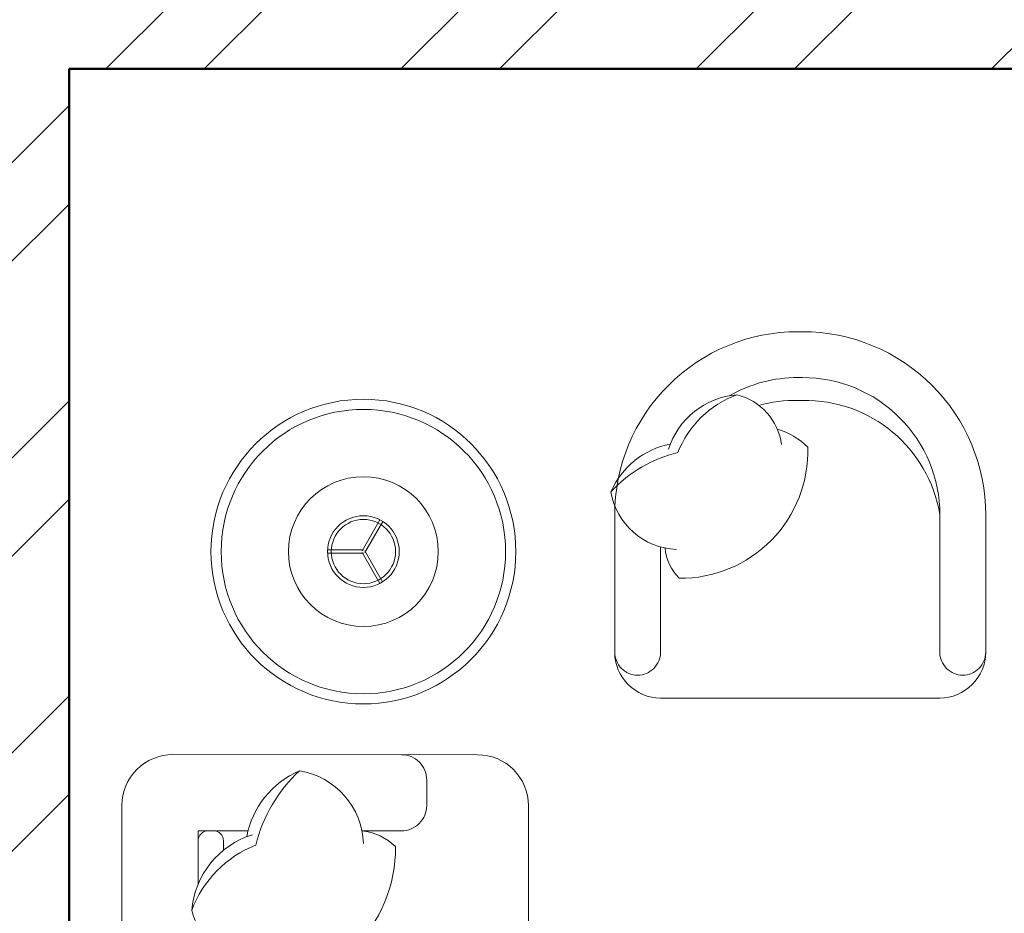
# Model space of a CAD drawing. Units: inches. Extents: x 963 to 2075, y 289 to 2657.
# Tile 85 of 98: x 1511 to 1556, y 2284 to 2325. Entities that reach past the tile are written whole.
import ezdxf

# ---------------------------------------------------------------- set-up
doc = ezdxf.new("R2010")
doc.units = ezdxf.units.IN
for name, color, linetype, lineweight in [('A-FURN', 8, 'Continuous', 18), ('A-WALL', 7, 'Continuous', 50), ('A-WALL-PATT', 8, 'Continuous', 13)]:
    doc.layers.add(name, color=color, linetype=linetype, lineweight=lineweight)

# ---------------------------------------------------------------- blocks, each defined once
blk = doc.blocks.new('SOFA-3SEAT')
at = {"ltscale": 0.03}
for p, q in [((7.593, 74.329), (6.776, 75.745)), ((7.719, 74.402), (6.902, 75.818)), ((7.593, 74.402), (6.776, 72.987)), ((7.719, 74.329), (6.902, 72.914)), ((7.656, 74.439), (9.29, 74.439)), ((7.656, 74.293), (9.29, 74.293)), ((7.719, 7.192), (6.902, 8.607)), ((7.593, 7.119), (6.776, 8.534)), ((7.593, 7.192), (6.776, 5.776)), ((7.656, 7.228), (9.29, 7.228)), ((7.719, 7.119), (6.902, 5.703)), ((7.656, 7.082), (9.29, 7.082))]:
    blk.add_line(p, q, dxfattribs=at)
blk.add_lwpolyline([(2.442, 16.426, -0.414214), (0.124, 18.743), (0.124, 32.649, -0.414214), (1.283, 33.808, -0.414214), (0.124, 34.967), (0.124, 46.555, -0.414214), (1.283, 47.713, -0.414214), (0.124, 48.872), (0.124, 62.778, -0.414214), (2.442, 65.095), (16.347, 65.095, -0.414214), (18.665, 62.778), (18.665, 18.743, -0.414214), (16.347, 16.426)], format="xyb", close=True, dxfattribs=at)
for points in [[(7.713, 61.619), (5.918, 61.619, -0.414214), (4.759, 62.778), (4.759, 63.937, -0.414214), (5.918, 65.095)], [(7.643, 61.038, -0.356772), (10.564, 64.358, -0.249542), (12.971, 61.349, 9.61688)], [(10.564, 64.358, -0.14773), (12.556, 60.971, -0.213343), (15.477, 57.983, -0.178662)], [(7.714, 61.622, 0.165541), (6.183, 60.905, 0.200231), (8.048, 56.305, 0.121523)], [(15.189, 59.181), (15.189, 61.619), (12.911, 61.619, -0.414214)], [(14.03, 60.735), (14.03, 61.156, -0.414214), (14.493, 61.619), (14.725, 61.619, -0.414214), (15.189, 61.156)], [(12.714, 61.439, -0.306663), (15.477, 57.983, -0.30633), (12.954, 55.725, 0.872847)], [(15.189, 61.156), (15.189, 59.181, -0.414214)], [(7.643, 54.795, -0.356772), (10.564, 58.116, -0.249542), (12.971, 55.107, 9.61688)], [(10.564, 58.116, -0.14773), (12.556, 54.729, -0.213343), (15.477, 51.74, -0.178662)], [(15.189, 57.253), (15.189, 52.939, -0.414214)], [(13.283, 54.97, 0.071865), (13.736, 55.942, -7.115464)], [(14.03, 54.492), (14.03, 56.087, -0.414214)], [(7.714, 55.379, 0.165541), (6.183, 54.662, 0.425989), (12.821, 48.154, 0.121523), (13.736, 49.699, -7.115464)], [(12.714, 55.197, -0.306663), (15.477, 51.74, -0.30633), (12.954, 49.482, 0.872847)], [(15.189, 51.011), (15.189, 48.177, -0.414214), (14.725, 47.713), (14.493, 47.713, -0.414214), (14.03, 48.177), (14.03, 49.844, -0.414214)], [(14.03, 48.872, -0.414214), (12.871, 47.713), (1.283, 47.713, -0.414214)], [(14.03, 46.555, 0.414214), (12.871, 47.713)], [(14.03, 34.967, -0.414214), (12.871, 33.808)], [(14.03, 32.649, 0.414214), (12.871, 33.808), (1.283, 33.808, 0.414214)], [(15.189, 24.268), (15.189, 33.344, 0.414214), (14.725, 33.808), (14.493, 33.808, 0.414214), (14.03, 33.344), (14.03, 25.435, 0.414214)], [(7.714, 19.9, -0.165541), (6.183, 20.616, -0.425989), (12.821, 27.124, -0.121523), (13.736, 25.58, 7.115464)], [(12.714, 20.082, 0.306663), (15.477, 23.538, 0.30633), (12.954, 25.796, -0.872847)], [(10.564, 17.163, 0.14773), (12.556, 20.55, 0.213343), (15.477, 23.538, 0.178662)], [(15.189, 20.366), (15.189, 22.34, 0.414214)], [(14.03, 20.786), (14.03, 20.366, 0.414214), (14.493, 19.902), (14.725, 19.902, 0.414214), (15.189, 20.366)], [(7.643, 20.484, 0.356772), (10.564, 17.163, 0.249542), (12.971, 20.172, -9.61688)], [(5.918, 16.426, -0.414214), (4.759, 17.584), (4.759, 18.743, -0.414214), (5.918, 19.902), (7.713, 19.902)]]:
    blk.add_lwpolyline(points, format="xyb")
for points in [[(15.189, 52.939), (15.189, 57.253)], [(15.189, 24.268), (15.189, 51.011)], [(12.911, 19.902), (15.189, 19.902), (15.189, 22.34)]]:
    blk.add_lwpolyline(points)
blk.add_lwpolyline([(15.189, 47.25), (15.189, 34.271, -0.414214), (14.725, 33.808), (14.493, 33.808, -0.414214), (14.03, 34.271), (14.03, 47.25, -0.414214), (14.493, 47.713), (14.725, 47.713, -0.414214)], format="xyb", close=True)
for centre, radius in [((7.656, 74.366), 6.953), ((7.656, 74.366), 3.418), ((7.656, 74.366), 1.636), ((7.656, 74.366), 1.466), ((7.656, 7.155), 6.953), ((7.656, 7.155), 3.418), ((7.656, 7.155), 1.636), ((7.656, 7.155), 1.466)]:
    blk.add_circle(centre, radius, dxfattribs=at)
for centre in [(7.656, 74.366), (7.656, 7.155)]:
    blk.add_circle(centre, 6.489)

msp = doc.modelspace()

# ---------------------------------------------------------------- hatches: boundary and pattern name
at = {"layer": 'A-WALL-PATT'}
h = msp.add_hatch(dxfattribs=at)
h.set_pattern_fill('ANSI32', color=256)
h.paths.add_polyline_path([(1296.922, 2558.318), (1203.922, 2558.318), (1203.922, 2493.818), (1191.533, 2493.818), (1191.533, 2489.318), (1211.063, 2489.318), (1211.063, 2492.02), (1211.063, 2493.818), (1208.422, 2493.818), (1208.422, 2553.818), (1292.422, 2553.818), (1292.422, 2538.863), (1296.922, 2538.863)])
h.paths.add_polyline_path([(1442.422, 2558.318), (1349.422, 2558.318), (1349.422, 2538.943), (1353.922, 2538.943), (1353.922, 2553.818), (1437.922, 2553.818), (1437.922, 2493.818), (1434.542, 2493.818), (1434.542, 2489.318), (1448.311, 2489.318), (1448.311, 2491.568), (1448.311, 2493.818), (1442.422, 2493.818)])
h.paths.add_polyline_path([(1415.554, 2491.568), (1415.554, 2493.818), (1340.941, 2493.818), (1340.941, 2489.318), (1371.922, 2489.318), (1371.922, 2378.318), (1367.596, 2378.318), (1367.596, 2373.818), (1371.922, 2373.818), (1371.922, 2355.185), (1376.422, 2355.185), (1376.422, 2489.318), (1415.554, 2489.318)])
h.paths.add_polyline_path([(1304.941, 2491.568), (1304.941, 2493.818), (1296.922, 2493.818), (1296.922, 2514.863), (1292.422, 2514.863), (1292.422, 2493.818), (1232.808, 2493.818), (1232.808, 2489.318), (1256.422, 2489.318), (1256.422, 2327.318), (1253.714, 2327.318), (1253.714, 2322.818), (1328.422, 2322.818), (1328.422, 2331.147), (1323.922, 2331.147), (1323.922, 2327.318), (1260.922, 2327.318), (1260.922, 2373.818), (1323.922, 2373.818), (1323.922, 2357.812), (1328.422, 2357.812), (1328.422, 2373.818), (1346.007, 2373.818), (1346.007, 2376.068), (1346.007, 2378.318), (1260.922, 2378.318), (1260.922, 2489.318), (1304.941, 2489.318)])
h.paths.add_polyline_path([(1226.654, 2327.318), (1124.422, 2327.318), (1124.422, 2347.447), (1119.922, 2347.447), (1119.922, 2322.818), (1163.422, 2322.818), (1163.422, 2305.435), (1165.672, 2305.435), (1167.922, 2305.435), (1167.922, 2322.818), (1226.654, 2322.818), (1226.654, 2325.068)])
h.paths.add_polyline_path([(1095.922, 2489.318), (1124.422, 2489.318), (1131.533, 2489.318), (1131.533, 2491.568), (1131.533, 2493.818), (1119.922, 2493.818), (1091.422, 2493.818), (1091.422, 2417.318), (1095.922, 2417.318), (1119.922, 2417.318), (1119.922, 2407.447), (1124.422, 2407.447), (1124.422, 2421.818), (1095.922, 2421.818)])
h.paths.add_polyline_path([(1512.922, 2558.318), (1508.422, 2558.318), (1508.422, 2493.818), (1503.401, 2493.818), (1503.401, 2489.318), (1508.422, 2489.318), (1508.422, 2327.318), (1376.422, 2327.318), (1376.422, 2330.273), (1371.922, 2330.273), (1371.922, 2298.744), (1376.422, 2298.744), (1376.422, 2322.818), (1508.422, 2322.818), (1508.422, 2165.318), (1504.255, 2165.318), (1504.255, 2160.818), (1508.422, 2160.818), (1508.422, 2108.318), (1512.922, 2108.318), (1512.922, 2160.818), (1516.182, 2160.818), (1516.182, 2163.068), (1516.182, 2165.318), (1512.922, 2165.318), (1512.922, 2322.818), (1644.922, 2322.818), (1644.922, 2298.744), (1649.422, 2298.744), (1649.422, 2322.818), (1649.422, 2330.944), (1647.172, 2330.944), (1644.922, 2330.944), (1644.922, 2327.318), (1512.922, 2327.318), (1512.922, 2489.318), (1516.759, 2489.318), (1516.759, 2491.568), (1516.759, 2493.818), (1512.922, 2493.818)])
h.paths.add_polyline_path([(1671.922, 2558.318), (1578.922, 2558.318), (1578.922, 2493.818), (1573.526, 2493.818), (1573.526, 2489.318), (1586.537, 2489.318), (1586.537, 2491.568), (1586.537, 2493.818), (1583.422, 2493.818), (1583.422, 2553.818), (1667.422, 2553.818), (1667.422, 2541.109), (1671.922, 2541.109)])
h.paths.add_polyline_path([(1681.257, 2493.818), (1671.922, 2493.818), (1671.922, 2517.109), (1667.422, 2517.109), (1667.422, 2493.818), (1610.218, 2493.818), (1610.218, 2489.318), (1644.922, 2489.318), (1644.922, 2357.865), (1649.422, 2357.865), (1649.422, 2373.818), (1652.203, 2373.818), (1652.203, 2375.827), (1652.203, 2378.318), (1649.422, 2378.318), (1649.422, 2489.318), (1681.257, 2489.318), (1681.257, 2491.568)])
h.paths.add_polyline_path([(1821.922, 2558.318), (1728.922, 2558.318), (1728.922, 2541), (1733.422, 2541), (1733.422, 2553.818), (1817.422, 2553.818), (1817.422, 2493.818), (1813.507, 2493.818), (1813.507, 2489.318), (1830.078, 2489.318), (1830.078, 2491.568), (1830.078, 2493.818), (1821.922, 2493.818)])
h.paths.add_polyline_path([(1794.244, 2493.818), (1717.257, 2493.818), (1717.257, 2489.318), (1760.422, 2489.318), (1760.422, 2378.318), (1674.401, 2378.318), (1674.401, 2373.818), (1692.922, 2373.818), (1692.922, 2356.954), (1697.422, 2356.954), (1697.422, 2373.818), (1760.422, 2373.818), (1760.422, 2327.318), (1697.422, 2327.318), (1697.422, 2333.341), (1692.922, 2333.341), (1692.922, 2322.818), (1768.037, 2322.818), (1768.037, 2325.068), (1768.037, 2327.318), (1764.922, 2327.318), (1764.922, 2489.318), (1794.244, 2489.318)])
h.paths.add_polyline_path([(1733.422, 2517), (1728.922, 2517), (1728.922, 2493.818), (1733.422, 2493.818)], flags=17)
h.paths.add_polyline_path([(1929.922, 2493.818), (1890.078, 2493.818), (1890.078, 2489.318), (1896.922, 2489.318), (1925.422, 2489.318), (1925.422, 2421.818), (1896.922, 2421.818), (1896.922, 2408.318), (1901.422, 2408.318), (1901.422, 2417.318), (1925.422, 2417.318), (1929.922, 2417.318)])
h.paths.add_polyline_path([(1901.422, 2348.318), (1896.922, 2348.318), (1896.922, 2327.318), (1800.423, 2327.318), (1800.423, 2322.818), (1853.422, 2322.818), (1853.422, 2309.453), (1857.922, 2309.453), (1857.922, 2322.818), (1901.422, 2322.818)])
h.paths.add_polyline_path([(1857.922, 2249.453), (1853.422, 2249.453), (1853.422, 2214.818), (1686.309, 2214.818), (1686.309, 2210.318), (1853.422, 2210.318), (1853.422, 2202.134), (1857.922, 2202.134), (1857.922, 2210.318)])
h.paths.add_polyline_path([(1857.922, 2142.134), (1853.422, 2142.134), (1853.422, 2115.422), (1841.422, 2115.422), (1841.422, 2088.531), (1841.422, 2046.949), (1845.922, 2046.949), (1845.922, 2110.922), (1905.922, 2110.922), (1905.922, 2092.517), (1910.422, 2092.517), (1910.422, 2115.422), (1857.922, 2115.422)])
h.paths.add_polyline_path([(1532.436, 1482.342), (1573.456, 1482.342), (1573.456, 1501), (1532.436, 1501)], flags=9)
h.paths.add_polyline_path([(1438.658, 1486.302), (1479.678, 1486.302), (1479.678, 1504.96), (1438.658, 1504.96)], flags=9)
h.paths.add_polyline_path([(1411.215, 1365.308), (1659.139, 1365.308), (1659.139, 1402.401), (1411.215, 1402.401)], flags=9)
h.paths.add_polyline_path([(1185.671, 2296.298), (1248.16, 2296.298), (1248.16, 2314.955), (1185.671, 2314.955)], flags=9)
h.paths.add_polyline_path([(1177.31, 2187.35), (1216.15, 2187.35), (1216.15, 2206.007), (1177.31, 2206.007)], flags=9)
h.paths.add_polyline_path([(1295.101, 1602.083), (1328.26, 1602.083), (1328.26, 1620.741), (1295.101, 1620.741)], flags=9)
h.paths.add_polyline_path([(1525.126, 2005.99), (1558.39, 2005.99), (1558.39, 2024.648), (1525.126, 2024.648)], flags=9)
h.paths.add_polyline_path([(1459.606, 1977.125), (1472.195, 1977.125), (1472.195, 1987.429), (1459.606, 1987.429)], flags=9)
h.paths.add_polyline_path([(1467.815, 2053.676), (1480.018, 2053.676), (1480.018, 2063.979), (1467.815, 2063.979)], flags=9)
h.paths.add_polyline_path([(1555.184, 2119.02), (1584.563, 2119.02), (1584.563, 2137.678), (1555.184, 2137.678)], flags=25)
h.paths.add_polyline_path([(1405.389, 2115.291), (1444.478, 2115.291), (1444.478, 2133.948), (1405.389, 2133.948)], flags=25)
h.paths.add_polyline_path([(1698.482, 2004.259), (1727.695, 2004.259), (1727.695, 2022.916), (1698.482, 2022.916)], flags=9)
h.paths.add_polyline_path([(1612.158, 1972.855), (1629.016, 1972.855), (1629.016, 1983.159), (1612.158, 1983.159)], flags=9)
h.paths.add_polyline_path([(1608.289, 2060.036), (1625.147, 2060.036), (1625.147, 2070.34), (1608.289, 2070.34)], flags=9)
h.paths.add_polyline_path([(1527.954, 1684.402), (1566.795, 1684.402), (1566.795, 1703.06), (1527.954, 1703.06)], flags=9)
h.paths.add_polyline_path([(1422.792, 1683.59), (1461.633, 1683.59), (1461.633, 1702.247), (1422.792, 1702.247)], flags=9)
h.paths.add_polyline_path([(1531.262, 1732.459), (1574.015, 1732.459), (1574.015, 1751.116), (1531.262, 1751.116)], flags=9)
h.paths.add_polyline_path([(1402.872, 1732.845), (1439.799, 1732.845), (1439.799, 1751.502), (1402.872, 1751.502)], flags=9)
h.paths.add_polyline_path([(1243.122, 1923.132), (1281.962, 1923.132), (1281.962, 1941.79), (1243.122, 1941.79)], flags=9)
h.paths.add_polyline_path([(1181.752, 1792.268), (1244.241, 1792.268), (1244.241, 1810.926), (1181.752, 1810.926)], flags=9)
h.paths.add_polyline_path([(1265.822, 1670.3), (1316.071, 1670.3), (1316.071, 1688.957), (1265.822, 1688.957)], flags=9)
h.paths.add_polyline_path([(1140.263, 1676.054), (1179.104, 1676.054), (1179.104, 1694.711), (1140.263, 1694.711)], flags=9)
h.paths.add_polyline_path([(1107.49, 1490.889), (1143.374, 1490.889), (1143.374, 1509.546), (1107.49, 1509.546)], flags=9)
h.paths.add_polyline_path([(1217.584, 1483.899), (1246.741, 1483.899), (1246.741, 1502.556), (1217.584, 1502.556)], flags=9)
h.paths.add_polyline_path([(1389.21, 1486.919), (1418.367, 1486.919), (1418.367, 1505.576), (1389.21, 1505.576)], flags=9)
h.paths.add_polyline_path([(1672.208, 1602.083), (1705.366, 1602.083), (1705.366, 1620.741), (1672.208, 1620.741)], flags=9)
h.paths.add_polyline_path([(1752.082, 1522.638), (1781.24, 1522.638), (1781.24, 1541.295), (1752.082, 1541.295)], flags=9)
h.paths.add_polyline_path([(1848.275, 1491.26), (1884.158, 1491.26), (1884.158, 1509.918), (1848.275, 1509.918)], flags=9)
h.paths.add_polyline_path([(1822.47, 1685.62), (1861.31, 1685.62), (1861.31, 1704.278), (1822.47, 1704.278)], flags=9)
h.paths.add_polyline_path([(1713.195, 1672.232), (1763.444, 1672.232), (1763.444, 1690.889), (1713.195, 1690.889)], flags=9)
h.paths.add_polyline_path([(1736.619, 1790.578), (1799.109, 1790.578), (1799.109, 1809.235), (1736.619, 1809.235)], flags=9)
h.paths.add_polyline_path([(1691.491, 1916.355), (1730.332, 1916.355), (1730.332, 1935.013), (1691.491, 1935.013)], flags=9)
h.paths.add_polyline_path([(1764.872, 1973.922), (1794.306, 1973.922), (1794.306, 1992.58), (1764.872, 1992.58)], flags=9)
h.paths.add_polyline_path([(1767.854, 2034.017), (1797.288, 2034.017), (1797.288, 2052.674), (1767.854, 2052.674)], flags=9)
h.paths.add_polyline_path([(1851.593, 2060.331), (1880.751, 2060.331), (1880.751, 2078.989), (1851.593, 2078.989)], flags=25)
h.paths.add_polyline_path([(1688.491, 2086.874), (1727.332, 2086.874), (1727.332, 2105.531), (1688.491, 2105.531)], flags=9)
h.paths.add_polyline_path([(1537.743, 2293.581), (1580.495, 2293.581), (1580.495, 2312.239), (1537.743, 2312.239)], flags=25)
h.paths.add_polyline_path([(1425.587, 2296.109), (1468.34, 2296.109), (1468.34, 2314.766), (1425.587, 2314.766)], flags=25)
h.paths.add_polyline_path([(1278.518, 2004.184), (1307.72, 2004.184), (1307.72, 2022.841), (1278.518, 2022.841)], flags=9)
h.paths.add_polyline_path([(1193.282, 1973.635), (1222.715, 1973.635), (1222.715, 1992.292), (1193.282, 1992.292)], flags=9)
h.paths.add_polyline_path([(1192.411, 2040.577), (1221.845, 2040.577), (1221.845, 2059.234), (1192.411, 2059.234)], flags=9)
h.paths.add_polyline_path([(1130.603, 1951.393), (1159.76, 1951.393), (1159.76, 1970.05), (1130.603, 1970.05)], flags=9)
h.paths.add_polyline_path([(1132.827, 2052.494), (1161.984, 2052.494), (1161.984, 2071.151), (1132.827, 2071.151)], flags=9)
h.paths.add_polyline_path([(1265.128, 2334.619), (1315.377, 2334.619), (1315.377, 2353.277), (1265.128, 2353.277)], flags=25)
h.paths.add_polyline_path([(1136.741, 2330.785), (1175.582, 2330.785), (1175.582, 2349.443), (1136.741, 2349.443)], flags=9)
h.paths.add_polyline_path([(1287.422, 2417.204), (1320.58, 2417.204), (1320.58, 2435.861), (1287.422, 2435.861)], flags=25)
h.paths.add_polyline_path([(1430.988, 2329.159), (1469.828, 2329.159), (1469.828, 2347.816), (1430.988, 2347.816)], flags=25)
h.paths.add_polyline_path([(1525.424, 2329.213), (1564.264, 2329.213), (1564.264, 2347.87), (1525.424, 2347.87)], flags=25)
h.paths.add_polyline_path([(1684.525, 2382.799), (1717.683, 2382.799), (1717.683, 2401.457), (1684.525, 2401.457)], flags=25)
h.paths.add_polyline_path([(1704.805, 2340.293), (1755.054, 2340.293), (1755.054, 2358.95), (1704.805, 2358.95)], flags=25)
h.paths.add_polyline_path([(1694.113, 2287.757), (1756.602, 2287.757), (1756.602, 2306.414), (1694.113, 2306.414)], flags=9)
h.paths.add_polyline_path([(1815.778, 2329.861), (1854.618, 2329.861), (1854.618, 2348.518), (1815.778, 2348.518)], flags=9)
h.paths.add_polyline_path([(1842.873, 2514.256), (1878.756, 2514.256), (1878.756, 2532.914), (1842.873, 2532.914)], flags=9)
h.paths.add_polyline_path([(1769.513, 2531.447), (1798.671, 2531.447), (1798.671, 2550.104), (1769.513, 2550.104)], flags=25)
h.paths.add_polyline_path([(1594.772, 2518.468), (1623.93, 2518.468), (1623.93, 2537.125), (1594.772, 2537.125)], flags=25)
h.paths.add_polyline_path([(1520.723, 2516.185), (1556.606, 2516.185), (1556.606, 2534.842), (1520.723, 2534.842)], flags=25)
h.paths.add_polyline_path([(1464.456, 2516.694), (1500.34, 2516.694), (1500.34, 2535.351), (1464.456, 2535.351)], flags=25)
h.paths.add_polyline_path([(1365.696, 2528.97), (1394.854, 2528.97), (1394.854, 2547.627), (1365.696, 2547.627)], flags=25)
h.paths.add_polyline_path([(1222.838, 2516.231), (1251.995, 2516.231), (1251.995, 2534.889), (1222.838, 2534.889)], flags=25)
h.paths.add_polyline_path([(1104.545, 2509.6), (1140.429, 2509.6), (1140.429, 2528.257), (1104.545, 2528.257)], flags=9)
h = msp.add_hatch(dxfattribs=at)
h.set_pattern_fill('ANSI32', color=256)
h.paths.add_polyline_path([(1335.968, 2212.568), (1335.968, 2214.818), (1167.922, 2214.818), (1167.922, 2245.435), (1163.422, 2245.435), (1163.422, 2210.318), (1163.422, 2194.812), (1167.922, 2194.812), (1167.922, 2210.318), (1335.968, 2210.318)])
h.paths.add_polyline_path([(1532.436, 1482.342), (1573.456, 1482.342), (1573.456, 1501), (1532.436, 1501)], flags=9)
h.paths.add_polyline_path([(1438.658, 1486.302), (1479.678, 1486.302), (1479.678, 1504.96), (1438.658, 1504.96)], flags=9)
h.paths.add_polyline_path([(1411.215, 1365.308), (1659.139, 1365.308), (1659.139, 1402.401), (1411.215, 1402.401)], flags=9)
h.paths.add_polyline_path([(1185.671, 2296.298), (1248.16, 2296.298), (1248.16, 2314.955), (1185.671, 2314.955)], flags=9)
h.paths.add_polyline_path([(1177.31, 2187.35), (1216.15, 2187.35), (1216.15, 2206.007), (1177.31, 2206.007)], flags=9)
h.paths.add_polyline_path([(1295.101, 1602.083), (1328.26, 1602.083), (1328.26, 1620.741), (1295.101, 1620.741)], flags=9)
h.paths.add_polyline_path([(1525.126, 2005.99), (1558.39, 2005.99), (1558.39, 2024.648), (1525.126, 2024.648)], flags=9)
h.paths.add_polyline_path([(1459.606, 1977.125), (1472.195, 1977.125), (1472.195, 1987.429), (1459.606, 1987.429)], flags=9)
h.paths.add_polyline_path([(1467.815, 2053.676), (1480.018, 2053.676), (1480.018, 2063.979), (1467.815, 2063.979)], flags=9)
h.paths.add_polyline_path([(1555.184, 2119.02), (1584.563, 2119.02), (1584.563, 2137.678), (1555.184, 2137.678)], flags=9)
h.paths.add_polyline_path([(1405.389, 2115.291), (1444.478, 2115.291), (1444.478, 2133.948), (1405.389, 2133.948)], flags=9)
h.paths.add_polyline_path([(1698.482, 2004.259), (1727.695, 2004.259), (1727.695, 2022.916), (1698.482, 2022.916)], flags=9)
h.paths.add_polyline_path([(1612.158, 1972.855), (1629.016, 1972.855), (1629.016, 1983.159), (1612.158, 1983.159)], flags=9)
h.paths.add_polyline_path([(1608.289, 2060.036), (1625.147, 2060.036), (1625.147, 2070.34), (1608.289, 2070.34)], flags=9)
h.paths.add_polyline_path([(1527.954, 1684.402), (1566.795, 1684.402), (1566.795, 1703.06), (1527.954, 1703.06)], flags=9)
h.paths.add_polyline_path([(1422.792, 1683.59), (1461.633, 1683.59), (1461.633, 1702.247), (1422.792, 1702.247)], flags=9)
h.paths.add_polyline_path([(1531.262, 1732.459), (1574.015, 1732.459), (1574.015, 1751.116), (1531.262, 1751.116)], flags=9)
h.paths.add_polyline_path([(1402.872, 1732.845), (1439.799, 1732.845), (1439.799, 1751.502), (1402.872, 1751.502)], flags=9)
h.paths.add_polyline_path([(1243.122, 1923.132), (1281.962, 1923.132), (1281.962, 1941.79), (1243.122, 1941.79)], flags=9)
h.paths.add_polyline_path([(1181.752, 1792.268), (1244.241, 1792.268), (1244.241, 1810.926), (1181.752, 1810.926)], flags=9)
h.paths.add_polyline_path([(1265.822, 1670.3), (1316.071, 1670.3), (1316.071, 1688.957), (1265.822, 1688.957)], flags=9)
h.paths.add_polyline_path([(1140.263, 1676.054), (1179.104, 1676.054), (1179.104, 1694.711), (1140.263, 1694.711)], flags=9)
h.paths.add_polyline_path([(1107.49, 1490.889), (1143.374, 1490.889), (1143.374, 1509.546), (1107.49, 1509.546)], flags=9)
h.paths.add_polyline_path([(1217.584, 1483.899), (1246.741, 1483.899), (1246.741, 1502.556), (1217.584, 1502.556)], flags=9)
h.paths.add_polyline_path([(1389.21, 1486.919), (1418.367, 1486.919), (1418.367, 1505.576), (1389.21, 1505.576)], flags=9)
h.paths.add_polyline_path([(1672.208, 1602.083), (1705.366, 1602.083), (1705.366, 1620.741), (1672.208, 1620.741)], flags=9)
h.paths.add_polyline_path([(1752.082, 1522.638), (1781.24, 1522.638), (1781.24, 1541.295), (1752.082, 1541.295)], flags=9)
h.paths.add_polyline_path([(1848.275, 1491.26), (1884.158, 1491.26), (1884.158, 1509.918), (1848.275, 1509.918)], flags=9)
h.paths.add_polyline_path([(1822.47, 1685.62), (1861.31, 1685.62), (1861.31, 1704.278), (1822.47, 1704.278)], flags=9)
h.paths.add_polyline_path([(1713.195, 1672.232), (1763.444, 1672.232), (1763.444, 1690.889), (1713.195, 1690.889)], flags=9)
h.paths.add_polyline_path([(1736.619, 1790.578), (1799.109, 1790.578), (1799.109, 1809.235), (1736.619, 1809.235)], flags=9)
h.paths.add_polyline_path([(1691.491, 1916.355), (1730.332, 1916.355), (1730.332, 1935.013), (1691.491, 1935.013)], flags=9)
h.paths.add_polyline_path([(1764.872, 1973.922), (1794.306, 1973.922), (1794.306, 1992.58), (1764.872, 1992.58)], flags=9)
h.paths.add_polyline_path([(1767.854, 2034.017), (1797.288, 2034.017), (1797.288, 2052.674), (1767.854, 2052.674)], flags=9)
h.paths.add_polyline_path([(1851.593, 2060.331), (1880.751, 2060.331), (1880.751, 2078.989), (1851.593, 2078.989)], flags=9)
h.paths.add_polyline_path([(1688.491, 2086.874), (1727.332, 2086.874), (1727.332, 2105.531), (1688.491, 2105.531)], flags=9)
h.paths.add_polyline_path([(1537.743, 2293.581), (1580.495, 2293.581), (1580.495, 2312.239), (1537.743, 2312.239)], flags=9)
h.paths.add_polyline_path([(1425.587, 2296.109), (1468.34, 2296.109), (1468.34, 2314.766), (1425.587, 2314.766)], flags=9)
h.paths.add_polyline_path([(1278.518, 2004.184), (1307.72, 2004.184), (1307.72, 2022.841), (1278.518, 2022.841)], flags=9)
h.paths.add_polyline_path([(1193.282, 1973.635), (1222.715, 1973.635), (1222.715, 1992.292), (1193.282, 1992.292)], flags=9)
h.paths.add_polyline_path([(1192.411, 2040.577), (1221.845, 2040.577), (1221.845, 2059.234), (1192.411, 2059.234)], flags=9)
h.paths.add_polyline_path([(1130.603, 1951.393), (1159.76, 1951.393), (1159.76, 1970.05), (1130.603, 1970.05)], flags=9)
h.paths.add_polyline_path([(1132.827, 2052.494), (1161.984, 2052.494), (1161.984, 2071.151), (1132.827, 2071.151)], flags=9)
h.paths.add_polyline_path([(1265.128, 2334.619), (1315.377, 2334.619), (1315.377, 2353.277), (1265.128, 2353.277)], flags=9)
h.paths.add_polyline_path([(1136.741, 2330.785), (1175.582, 2330.785), (1175.582, 2349.443), (1136.741, 2349.443)], flags=9)
h.paths.add_polyline_path([(1287.422, 2417.204), (1320.58, 2417.204), (1320.58, 2435.861), (1287.422, 2435.861)], flags=9)
h.paths.add_polyline_path([(1430.988, 2329.159), (1469.828, 2329.159), (1469.828, 2347.816), (1430.988, 2347.816)], flags=9)
h.paths.add_polyline_path([(1525.424, 2329.213), (1564.264, 2329.213), (1564.264, 2347.87), (1525.424, 2347.87)], flags=9)
h.paths.add_polyline_path([(1684.525, 2382.799), (1717.683, 2382.799), (1717.683, 2401.457), (1684.525, 2401.457)], flags=9)
h.paths.add_polyline_path([(1704.805, 2340.293), (1755.054, 2340.293), (1755.054, 2358.95), (1704.805, 2358.95)], flags=9)
h.paths.add_polyline_path([(1694.113, 2287.757), (1756.602, 2287.757), (1756.602, 2306.414), (1694.113, 2306.414)], flags=9)
h.paths.add_polyline_path([(1815.778, 2329.861), (1854.618, 2329.861), (1854.618, 2348.518), (1815.778, 2348.518)], flags=9)
h.paths.add_polyline_path([(1842.873, 2514.256), (1878.756, 2514.256), (1878.756, 2532.914), (1842.873, 2532.914)], flags=9)
h.paths.add_polyline_path([(1769.513, 2531.447), (1798.671, 2531.447), (1798.671, 2550.104), (1769.513, 2550.104)], flags=9)
h.paths.add_polyline_path([(1594.772, 2518.468), (1623.93, 2518.468), (1623.93, 2537.125), (1594.772, 2537.125)], flags=9)
h.paths.add_polyline_path([(1520.723, 2516.185), (1556.606, 2516.185), (1556.606, 2534.842), (1520.723, 2534.842)], flags=9)
h.paths.add_polyline_path([(1464.456, 2516.694), (1500.34, 2516.694), (1500.34, 2535.351), (1464.456, 2535.351)], flags=9)
h.paths.add_polyline_path([(1365.696, 2528.97), (1394.854, 2528.97), (1394.854, 2547.627), (1365.696, 2547.627)], flags=9)
h.paths.add_polyline_path([(1222.838, 2516.231), (1251.995, 2516.231), (1251.995, 2534.889), (1222.838, 2534.889)], flags=9)
h.paths.add_polyline_path([(1104.545, 2509.6), (1140.429, 2509.6), (1140.429, 2528.257), (1104.545, 2528.257)], flags=9)

# ---------------------------------------------------------------- linework, layer by layer
at = {"layer": 'A-FURN', "ltscale": 0.03}
msp.add_lwpolyline([(1546.28, 2294.108), (1552.653, 2294.108, 0.414214), (1554.743, 2296.198), (1554.743, 2302.467, 0.414214), (1546.384, 2310.825), (1546.28, 2310.825), (1546.175, 2310.825, 0.414214), (1537.817, 2302.467), (1537.817, 2296.198, 0.414214), (1539.906, 2294.108), (1546.28, 2294.108)], format="xyb", dxfattribs=at)
at = {"layer": 'A-FURN'}
for points in [[(1543.063, 2307.909, -0.130591), (1546.175, 2308.736), (1546.28, 2308.736)], [(1552.653, 2302.467, 0.414214), (1546.384, 2308.736), (1546.28, 2308.736)], [(1537.646, 2303.521, -0.14773), (1540.699, 2305.317, -0.213343), (1543.394, 2307.95, -0.178662)], [(1540.278, 2305.46, -0.306663), (1543.394, 2307.95, -0.30633), (1545.43, 2305.676, 0.872847)], [(1544.394, 2307.466, -0.072384), (1546.175, 2307.691), (1546.28, 2307.691)], [(1552.653, 2302.467, 0.372719), (1546.384, 2307.691), (1546.28, 2307.691)], [(1540.113, 2300.951, 0.165541), (1540.759, 2299.571, 0.425989), (1546.627, 2305.556, 0.121523), (1545.234, 2306.381, -7.115464)], [(1540.64, 2300.888, -0.356772), (1537.646, 2303.521, -0.249542), (1540.358, 2305.692, 9.61688)], [(1552.653, 2302.467), (1552.653, 2296.198, 0.414214), (1553.698, 2295.153), (1553.698, 2295.153, 0.414214), (1554.743, 2296.198)], [(1539.906, 2301.002), (1539.906, 2296.198, -0.414214), (1538.861, 2295.153), (1538.861, 2295.153, -0.414214), (1537.817, 2296.198)]]:
    msp.add_lwpolyline(points, format="xyb", dxfattribs=at)
at = {"layer": 'A-WALL'}
for p, q in [((1512.922, 2322.818), (1644.922, 2322.818)), ((1512.922, 2165.318), (1512.922, 2322.818))]:
    msp.add_line(p, q, dxfattribs=at)

# ---------------------------------------------------------------- block references
at = {"layer": 'A-FURN', "rotation": 179.9690487318625}
msp.add_blockref('SOFA-3SEAT', (1534.012, 2307.942), dxfattribs=at)

doc.saveas('drawing.dxf')
